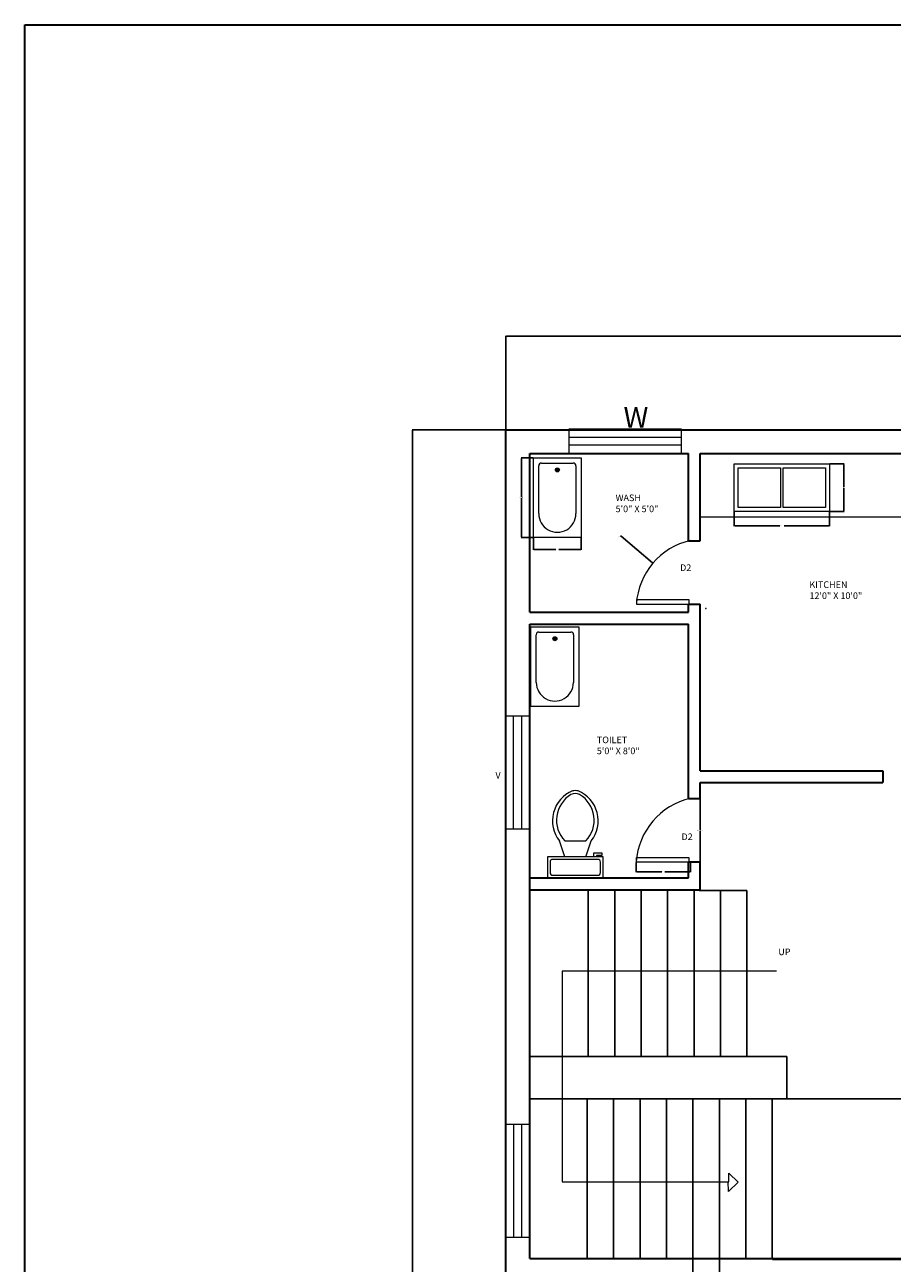
# Model space of a CAD drawing. Units: inches. Extents: x 65 to 1274, y 42 to 1041.
# Tile 2 of 6: x 65 to 393, y 573 to 1041. Entities that reach past the tile are written whole.
import ezdxf

# ---------------------------------------------------------------- set-up
doc = ezdxf.new("R2010")
doc.units = ezdxf.units.IN
for name, color, linetype, lineweight in [('A-ANNO-DIMS', 2, 'Continuous', 18), ('A-ANNO-SYMB', 7, 'Continuous', 13), ('A-AREA-IDEN', 7, 'Continuous', 18), ('A-DOOR', 3, 'Continuous', 18), ('A-FLOR-CASE', 8, 'Continuous', 18), ('A-FLOR-FIXT', 9, 'Continuous', 18), ('A-FLOR-STRS', 2, 'Continuous', 25), ('A-GLAZ', 4, 'Continuous', 18), ('A-WALL', 7, 'Continuous', 35), ('Text', 7, 'Continuous', 18), ('Title Block', 7, 'Continuous', 35)]:
    doc.layers.add(name, color=color, linetype=linetype, lineweight=lineweight)
doc.styles.get("Standard").update_dxf_attribs({"font": 'arial.ttf'})
doc.dimstyles.get("Standard").update_dxf_attribs({"dimtxt": 0.18, "dimasz": 0.18, "dimexe": 0.18, "dimexo": 0.0625, "dimgap": 0.09, "dimtad": 0, "dimtih": 1, "dimtoh": 1, "dimdec": 4, "dimzin": 0, "dimdsep": 46, "dimtxsty": 'Standard', "dimcen": 0.09, "dimadec": 0, "dimazin": 0, "dimtfac": 1, "dimtdec": 4, "dimtofl": 0, "dimtmove": 0, "dimatfit": 3, "dimfxl": 1, "dimtolj": 1, "dimtzin": 0, "dimarcsym": 0})

# ---------------------------------------------------------------- blocks, each defined once
blk = doc.blocks.new('Wall Cabinet - 18 x 36 in front')
for p, q in [((17.5, -1.5), (17.5, -16.5)), ((18.5, -16.5), (18.5, -1.5))]:
    blk.add_line(p, q)
blk.add_lwpolyline([(0, -18), (0, 0), (36, 0), (36, -18)], close=True)
for points in [[(17.5, -16.5), (1.5, -16.5), (1.5, -1.5), (17.5, -1.5)], [(18.5, -1.5), (34.5, -1.5), (34.5, -16.5), (18.5, -16.5)]]:
    blk.add_lwpolyline(points)
blk = doc.blocks.new('Bath Tub - 26 x 60 in.')
for p, q in [((8, -18), (10, -18)), ((9, -17), (9, -19))]:
    blk.add_line(p, q)
blk.add_lwpolyline([(0, -36), (0, 0), (60, 0), (60, -36)], close=True)
for points in [[(4, -30), (4, -6)], [(6, -4), (42, -4)], [(42, -32), (6, -32)]]:
    blk.add_lwpolyline(points)
for radius in [1.5, 1]:
    blk.add_circle((9, -18), radius)
for centre, radius, start, end in [((5.75, -5.75), 1.77, 81.8699, 188.1301), ((42, -18), 14, 270, 90), ((5.75, -30.25), 1.77, 171.8699, 278.1301)]:
    blk.add_arc(centre, radius, start, end)
blk = doc.blocks.new('Toilet - top')
for p, q in [((9.5, -6), (9.5, -2)), ((-10, -8.5), (-8, -8.5)), ((-10, -9.5), (-10, -8.5)), ((-8, -8.5), (-8, -8)), ((-7, -8), (-7, -9.5)), ((-4, -8), (-6, -14)), ((4, -8), (6, -14)), ((-7, -9.5), (-10, -9.5)), ((4, -14), (-4, -14))]:
    blk.add_line(p, q)
blk.add_lwpolyline([(10.5, -8), (10.5, 0), (-10.5, 0), (-10.5, -8)], close=True)
for points in [[(-9.5, -2), (-9.5, -6)], [(8.5, -1), (-8.5, -1)], [(-8.5, -7), (8.5, -7)]]:
    blk.add_lwpolyline(points)
for centre, radius, start, end in [((-8.62, -1.88), 0.884, 81.8699, 188.1301), ((8.62, -1.88), 0.884, 351.8699, 98.1301), ((-8.62, -6.12), 0.884, 171.8699, 278.1301), ((8.62, -6.12), 0.884, 261.8699, 8.1301), ((3.52, -21.58), 12.17, 141.4691, 247.9714), ((4.2, -21.82), 11.33, 136.3677, 238.9468), ((-3.52, -21.58), 12.17, 292.0284, 38.5307), ((-4.2, -21.82), 11.33, 301.053, 43.6321), ((0, -27.88), 4, 245.7318, 294.2682), ((0, -29), 4, 254.8605, 285.1395)]:
    blk.add_arc(centre, radius, start, end)
blk = doc.blocks.new('WIN-43-DEEP-FRAME')
for p, q in [((9, 42.65), (0, 42.65)), ((0, 42.65), (0, 0)), ((3, 0), (3, 42.65)), ((6, 42.65), (6, 0)), ((9, 0), (9, 42.65)), ((0, 0), (9, 0))]:
    blk.add_line(p, q)
blk = doc.blocks.new('DOOR-SINGLE-24')
blk.add_lwpolyline([(19.83, 0), (0.13, 0), (0.13, 1.84), (19.83, 1.84)], close=True)
blk.add_arc((26.27, -1.53), 26.32, 102.6921, 176.3801)
blk = doc.blocks.new('*D26')
at = {"layer": 'A-ANNO-DIMS', "color": 0, "lineweight": -2, "transparency": 16777216}
for p, q in [((316.53, 748.64), (320.27, 748.64)), ((320.09, 748.46), (320.09, 736.75)), ((320.09, 724.68), (320.09, 736.39)), ((316.53, 724.5), (320.27, 724.5))]:
    blk.add_line(p, q, dxfattribs=at)
at = {"layer": 'A-ANNO-DIMS', "color": 0, "transparency": 16777216}
for points in [[(320.06, 748.46), (320.12, 748.46), (320.09, 748.64)], [(320.06, 724.68), (320.12, 724.68), (320.09, 724.5)]]:
    blk.add_solid(points, dxfattribs=at)
at = {"layer": 'Defpoints', "color": 0, "transparency": 16777216}
for p in [(316.47, 748.64), (320.09, 748.64), (316.47, 724.5)]:
    blk.add_point(p, dxfattribs=at)
at = {"layer": 'A-ANNO-DIMS', "color": 0, "transparency": 16777216, "insert": (320.09, 736.57), "char_height": 0.18, "attachment_point": 5}
blk.add_mtext('\\A1;SERVICE DOOR 24 TYP.', dxfattribs=at)
blk = doc.blocks.new('*D27')
at = {"layer": 'A-ANNO-DIMS', "color": 0, "lineweight": -2, "transparency": 16777216}
for p, q in [((295.99, 724.44), (295.99, 720.7)), ((316.47, 724.44), (316.47, 720.7)), ((296.17, 720.88), (305.7, 720.88)), ((316.29, 720.88), (306.76, 720.88))]:
    blk.add_line(p, q, dxfattribs=at)
at = {"layer": 'A-ANNO-DIMS', "color": 0, "transparency": 16777216}
for points in [[(296.17, 720.91), (296.17, 720.85), (295.99, 720.88)], [(316.29, 720.91), (316.29, 720.85), (316.47, 720.88)]]:
    blk.add_solid(points, dxfattribs=at)
at = {"layer": 'Defpoints', "color": 0, "transparency": 16777216}
for p in [(295.99, 724.5), (316.47, 724.5), (316.47, 720.88)]:
    blk.add_point(p, dxfattribs=at)
at = {"layer": 'A-ANNO-DIMS', "color": 0, "transparency": 16777216, "insert": (306.23, 720.88), "char_height": 0.18, "attachment_point": 5}
blk.add_mtext('\\A1;20 TYP.', dxfattribs=at)
blk = doc.blocks.new('*D32')
at = {"layer": 'A-ANNO-DIMS', "color": 0, "lineweight": -2, "transparency": 16777216}
for p, q in [((257.04, 877.45), (252.4, 877.45)), ((252.58, 877.27), (252.58, 862.56)), ((252.58, 847.5), (252.58, 862.2)), ((257.04, 847.32), (252.4, 847.32))]:
    blk.add_line(p, q, dxfattribs=at)
at = {"layer": 'A-ANNO-DIMS', "color": 0, "transparency": 16777216}
for points in [[(252.55, 877.27), (252.61, 877.27), (252.58, 877.45)], [(252.55, 847.5), (252.61, 847.5), (252.58, 847.32)]]:
    blk.add_solid(points, dxfattribs=at)
at = {"layer": 'Defpoints', "color": 0, "transparency": 16777216}
for p in [(257.1, 877.45), (252.58, 847.32), (257.1, 847.32)]:
    blk.add_point(p, dxfattribs=at)
at = {"layer": 'A-ANNO-DIMS', "color": 0, "transparency": 16777216, "insert": (252.58, 862.38), "char_height": 0.18, "attachment_point": 5}
blk.add_mtext('\\A1;TUB 30 TYP.', dxfattribs=at)
blk = doc.blocks.new('*D33')
at = {"layer": 'A-ANNO-DIMS', "color": 0, "lineweight": -2, "transparency": 16777216}
for p, q in [((257.1, 847.25), (257.1, 842.62)), ((275.18, 847.25), (275.18, 842.62)), ((257.28, 842.8), (265.62, 842.8)), ((275, 842.8), (266.66, 842.8))]:
    blk.add_line(p, q, dxfattribs=at)
at = {"layer": 'A-ANNO-DIMS', "color": 0, "transparency": 16777216}
for points in [[(257.28, 842.83), (257.28, 842.77), (257.1, 842.8)], [(275, 842.83), (275, 842.77), (275.18, 842.8)]]:
    blk.add_solid(points, dxfattribs=at)
at = {"layer": 'Defpoints', "color": 0, "transparency": 16777216}
for p in [(257.1, 847.32), (275.18, 847.32), (275.18, 842.8)]:
    blk.add_point(p, dxfattribs=at)
at = {"layer": 'A-ANNO-DIMS', "color": 0, "transparency": 16777216, "insert": (266.14, 842.8), "char_height": 0.18, "attachment_point": 5}
blk.add_mtext('\\A1;18 TYP.', dxfattribs=at)
blk = doc.blocks.new('*D50')
at = {"layer": 'A-ANNO-DIMS', "color": 0, "lineweight": -2, "transparency": 16777216}
for p, q in [((333.04, 857.11), (333.04, 851.59)), ((369.04, 857.11), (369.04, 851.59)), ((333.22, 851.77), (350.25, 851.77)), ((368.86, 851.77), (351.84, 851.77))]:
    blk.add_line(p, q, dxfattribs=at)
at = {"layer": 'A-ANNO-DIMS', "color": 0, "transparency": 16777216}
for points in [[(333.22, 851.8), (333.22, 851.74), (333.04, 851.77)], [(368.86, 851.8), (368.86, 851.74), (369.04, 851.77)]]:
    blk.add_solid(points, dxfattribs=at)
at = {"layer": 'Defpoints', "color": 0, "transparency": 16777216}
for p in [(333.04, 857.17), (369.04, 857.17), (369.04, 851.77)]:
    blk.add_point(p, dxfattribs=at)
at = {"layer": 'A-ANNO-DIMS', "color": 0, "transparency": 16777216, "insert": (351.04, 851.77), "char_height": 0.18, "attachment_point": 5}
blk.add_mtext('\\A1;CABINET 36', dxfattribs=at)
blk = doc.blocks.new('*D51')
at = {"layer": 'A-ANNO-DIMS', "color": 0, "lineweight": -2, "transparency": 16777216}
for p, q in [((369.11, 875.17), (374.62, 875.17)), ((374.44, 874.99), (374.44, 866.35)), ((374.44, 857.35), (374.44, 865.99)), ((369.11, 857.17), (374.62, 857.17))]:
    blk.add_line(p, q, dxfattribs=at)
at = {"layer": 'A-ANNO-DIMS', "color": 0, "transparency": 16777216}
for points in [[(374.41, 874.99), (374.47, 874.99), (374.44, 875.17)], [(374.41, 857.35), (374.47, 857.35), (374.44, 857.17)]]:
    blk.add_solid(points, dxfattribs=at)
at = {"layer": 'Defpoints', "color": 0, "transparency": 16777216}
for p in [(369.04, 875.17), (374.44, 875.17), (369.04, 857.17)]:
    blk.add_point(p, dxfattribs=at)
at = {"layer": 'A-ANNO-DIMS', "color": 0, "transparency": 16777216, "insert": (374.44, 866.17), "char_height": 0.18, "attachment_point": 5}
blk.add_mtext('\\A1;18', dxfattribs=at)
blk = doc.blocks.new('*D52')
at = {"layer": 'A-ANNO-DIMS', "color": 0, "lineweight": -2, "transparency": 16777216}
for p, q in [((246.69, 888.16), (246.69, 923.68)), ((246.87, 923.5), (438.4, 923.5)), ((630.51, 923.5), (438.98, 923.5)), ((630.69, 888.16), (630.69, 923.68))]:
    blk.add_line(p, q, dxfattribs=at)
at = {"layer": 'A-ANNO-DIMS', "color": 0, "transparency": 16777216}
for points in [[(246.87, 923.53), (246.87, 923.47), (246.69, 923.5)], [(630.51, 923.53), (630.51, 923.47), (630.69, 923.5)]]:
    blk.add_solid(points, dxfattribs=at)
at = {"layer": 'Defpoints', "color": 0, "transparency": 16777216}
for p in [(630.69, 923.5), (246.69, 888.1), (630.69, 888.1)]:
    blk.add_point(p, dxfattribs=at)
at = {"layer": 'A-ANNO-DIMS', "color": 0, "transparency": 16777216, "insert": (438.69, 923.5), "char_height": 0.18, "attachment_point": 5}
blk.add_mtext('\\A1;384', dxfattribs=at)
blk = doc.blocks.new('*D53')
at = {"layer": 'A-ANNO-DIMS', "color": 0, "lineweight": -2, "transparency": 16777216}
for p, q in [((246.62, 888.1), (211.23, 888.1)), ((211.41, 887.92), (211.41, 559.78)), ((211.41, 231.28), (211.41, 559.42)), ((246.62, 231.1), (211.23, 231.1))]:
    blk.add_line(p, q, dxfattribs=at)
at = {"layer": 'A-ANNO-DIMS', "color": 0, "transparency": 16777216}
for points in [[(211.38, 887.92), (211.44, 887.92), (211.41, 888.1)], [(211.38, 231.28), (211.44, 231.28), (211.41, 231.1)]]:
    blk.add_solid(points, dxfattribs=at)
at = {"layer": 'Defpoints', "color": 0, "transparency": 16777216}
for p in [(211.41, 888.1), (246.69, 888.1), (246.69, 231.1)]:
    blk.add_point(p, dxfattribs=at)
at = {"layer": 'A-ANNO-DIMS', "color": 0, "transparency": 16777216, "insert": (211.41, 559.6), "char_height": 0.18, "attachment_point": 5}
blk.add_mtext('\\A1;657', dxfattribs=at)
blk = doc.blocks.new('*D62')
at = {"layer": 'A-ANNO-DIMS', "color": 0, "lineweight": -2, "transparency": 16777216}
for p, q in [((347.47, 635.01), (666.07, 635.01)), ((665.89, 634.83), (665.89, 604.83)), ((665.89, 574.45), (665.89, 604.46)), ((347.47, 574.27), (666.07, 574.27))]:
    blk.add_line(p, q, dxfattribs=at)
at = {"layer": 'A-ANNO-DIMS', "color": 0, "transparency": 16777216}
for points in [[(665.86, 634.83), (665.92, 634.83), (665.89, 635.01)], [(665.86, 574.45), (665.92, 574.45), (665.89, 574.27)]]:
    blk.add_solid(points, dxfattribs=at)
at = {"layer": 'Defpoints', "color": 0, "transparency": 16777216}
for p in [(347.41, 635.01), (665.89, 635.01), (347.41, 574.27)]:
    blk.add_point(p, dxfattribs=at)
at = {"layer": 'A-ANNO-DIMS', "color": 0, "transparency": 16777216, "insert": (665.89, 604.64), "char_height": 0.18, "attachment_point": 5}
blk.add_mtext('\\A1;60.74', dxfattribs=at)
blk = doc.blocks.new('*D63')
at = {"layer": 'A-ANNO-DIMS', "color": 0, "lineweight": -2, "transparency": 16777216}
for p, q in [((317.41, 574.21), (317.41, 195.72)), ((327.41, 574.21), (327.41, 195.72)), ((317.59, 195.9), (322.2, 195.9)), ((327.23, 195.9), (322.62, 195.9))]:
    blk.add_line(p, q, dxfattribs=at)
at = {"layer": 'A-ANNO-DIMS', "color": 0, "transparency": 16777216}
for points in [[(317.59, 195.93), (317.59, 195.87), (317.41, 195.9)], [(327.23, 195.93), (327.23, 195.87), (327.41, 195.9)]]:
    blk.add_solid(points, dxfattribs=at)
at = {"layer": 'Defpoints', "color": 0, "transparency": 16777216}
for p in [(317.41, 574.27), (327.41, 574.27), (327.41, 195.9)]:
    blk.add_point(p, dxfattribs=at)
at = {"layer": 'A-ANNO-DIMS', "color": 0, "transparency": 16777216, "insert": (322.41, 195.9), "char_height": 0.18, "attachment_point": 5}
blk.add_mtext('\\A1;10', dxfattribs=at)
blk = doc.blocks.new('*D79')
at = {"layer": 'A-ANNO-DIMS', "color": 0, "lineweight": -2, "transparency": 16777216}
for p, q in [((290.06, 847.85), (290.24, 847.85)), ((290.24, 847.85), (302.11, 837.72)), ((322.18, 820.52), (322.36, 820.52)), ((322.27, 820.43), (322.27, 820.61))]:
    blk.add_line(p, q, dxfattribs=at)
at = {"layer": 'A-ANNO-DIMS', "color": 0, "transparency": 16777216}
blk.add_solid([(302.13, 837.74), (302.09, 837.69), (302.25, 837.6)], dxfattribs=at)
at = {"layer": 'Defpoints', "color": 0, "transparency": 16777216}
for p in [(302.25, 837.6), (322.27, 820.52)]:
    blk.add_point(p, dxfattribs=at)
at = {"layer": 'A-ANNO-DIMS', "color": 0, "transparency": 16777216, "insert": (289.38, 847.85), "char_height": 0.18, "attachment_point": 5}
blk.add_mtext('\\A1;2X R26.32', dxfattribs=at)

msp = doc.modelspace()

# ---------------------------------------------------------------- linework, layer by layer
at = {"layer": 'A-ANNO-SYMB'}
for p, q in [((349.0318, 683.2572), (267.9966, 683.2572)), ((267.9966, 683.2572), (267.9966, 603.565)), ((330.9282, 603.565), (330.9282, 606.9116)), ((330.9282, 606.9116), (334.457, 603.5371)), ((267.9966, 603.565), (330.9282, 603.565)), ((330.9115, 599.9938), (330.7427, 603.7058)), ((334.457, 603.5371), (330.9115, 599.9938))]:
    msp.add_line(p, q, dxfattribs=at)
at = {"layer": 'A-FLOR-CASE'}
msp.add_line((320.1872, 855.1013), (440.1872, 855.1013), dxfattribs=at)
at = {"layer": 'A-FLOR-STRS'}
for p, q in [((277.8365, 713.8438), (277.8365, 650.9516)), ((287.8365, 713.8438), (287.8365, 650.9516)), ((297.8365, 713.8438), (297.8365, 650.9516)), ((307.8365, 713.8438), (307.8365, 650.9516)), ((317.8365, 713.8438), (317.8365, 650.9516)), ((319.7329, 713.8438), (337.8365, 713.8438)), ((327.8365, 713.8438), (327.8365, 650.9516)), ((337.8365, 713.8438), (337.8365, 650.9516)), ((255.6872, 650.9516), (352.9229, 650.9516)), ((352.9229, 650.9516), (352.9229, 635.0131)), ((352.9229, 635.0131), (255.6872, 635.0131)), ((277.4055, 635.0131), (277.4055, 574.2747)), ((287.4055, 635.0131), (287.4055, 574.2747)), ((297.4055, 635.0131), (297.4055, 574.2747)), ((307.4055, 635.0131), (307.4055, 574.2747)), ((317.4055, 635.0131), (317.4055, 574.2747)), ((327.4055, 635.0131), (327.4055, 574.2747)), ((337.4055, 635.0131), (337.4055, 574.2747)), ((347.4055, 635.0131), (347.4055, 574.2747))]:
    msp.add_line(p, q, dxfattribs=at)
at = {"layer": 'A-WALL'}
for p, q in [((246.6872, 231.1013), (246.6872, 888.1013)), ((246.6872, 888.1013), (630.6872, 888.1013)), ((255.6872, 879.1013), (315.6872, 879.1013)), ((255.6872, 819.1013), (255.6872, 879.1013)), ((315.6872, 846.1013), (315.6872, 879.1013)), ((315.6872, 846.1013), (315.6872, 879.1013)), ((320.1872, 846.1013), (320.1872, 879.1013)), ((320.1872, 879.1013), (464.1872, 879.1013)), ((315.6872, 846.1013), (320.1872, 846.1013)), ((315.6872, 819.1013), (315.6872, 822.1013)), ((315.6872, 822.1013), (320.1872, 822.1013)), ((315.6872, 819.1013), (315.6872, 822.1013)), ((320.1872, 759.1013), (320.1872, 822.1013)), ((255.6872, 819.1013), (315.6872, 819.1013)), ((320.1872, 814.6013), (320.1872, 819.1013)), ((255.6872, 814.6013), (315.6872, 814.6013)), ((255.6872, 574.6013), (255.6872, 814.6013)), ((315.6872, 748.6013), (315.6872, 814.6013)), ((320.1872, 759.1013), (389.1872, 759.1013)), ((389.1872, 759.1013), (389.1872, 754.6013)), ((320.1872, 754.6013), (389.1872, 754.6013)), ((320.1872, 748.6013), (320.1872, 754.6013)), ((315.6872, 748.6013), (320.1872, 748.6013)), ((315.6872, 718.6013), (315.6872, 724.6013)), ((315.6872, 724.6013), (320.1872, 724.6013)), ((320.1872, 714.1013), (320.1872, 724.6013)), ((255.6872, 718.6013), (315.6872, 718.6013)), ((255.6872, 714.1013), (320.1872, 714.1013)), ((255.6872, 574.6013), (441.6872, 574.6013))]:
    msp.add_line(p, q, dxfattribs=at)
at = {"layer": 'Title Block'}
msp.add_lwpolyline([(64.7421, 1041.286), (1273.976, 1041.286), (1273.976, 41.6396), (64.7421, 41.6396)], close=True, dxfattribs=at)

# ---------------------------------------------------------------- block references
at = {"layer": 'A-DOOR'}
for p in [(296.0064, 822.0505), (295.986, 724.499)]:
    msp.add_blockref('DOOR-SINGLE-24', p, dxfattribs=at)
at = {"layer": 'A-FLOR-CASE'}
msp.add_blockref('Wall Cabinet - 18 x 36 in front', (333.043, 875.1694), dxfattribs=at)
at = {"layer": 'A-FLOR-FIXT', "xscale": 0.5021616587859374, "yscale": 0.5021616587859374, "zscale": 0.5021616587859374, "rotation": 270}
for p in [(275.1788, 877.4464), (274.2366, 813.5706)]:
    msp.add_blockref('Bath Tub - 26 x 60 in.', p, dxfattribs=at)
at = {"layer": 'A-FLOR-FIXT', "rotation": 180}
msp.add_blockref('Toilet - top', (272.9251, 718.5865), dxfattribs=at)
at = {"layer": 'A-GLAZ'}
for p, rotation in [((270.476, 888.2993), 269.9999999999994), ((255.6126, 779.7517), 180), ((255.621, 625.3174), 180)]:
    msp.add_blockref('WIN-43-DEEP-FRAME', p, dxfattribs=dict(at, rotation=rotation))

# ---------------------------------------------------------------- texts
at = {"layer": 'A-AREA-IDEN', "char_height": 2.5, "attachment_point": 1}
for s, width, insert in [('WASH\\P5\'0" X 5\'0"', 20.053164, (288.1552, 863.5853)), ('KITCHEN\\P12\'0" X 10\'0"', 36.578531, (361.4522, 830.7528)), ('TOILET\\P5\'0" X 8\'0" ', 18.101103, (281.0621, 772.0325))]:
    msp.add_mtext_dynamic_manual_height_columns(s, width=width, gutter_width=12.5, heights=[0], dxfattribs=dict(at, insert=insert))
at = {"layer": 'Text', "attachment_point": 1}
for s, width, gutter_width, insert, char_height in [('W', 96.254197, 39.1027, (291.1598, 896.645), 7.8205), ('D2', 14.123415, 12.5, (312.5465, 837.1667), 2.5), ('V', 5.099062, 12.5, (242.7261, 758.6419), 2.5), ('D2', 14.019907, 12.5, (313.0605, 735.3946), 2.5), ('UP', 18.012995, 12.5, (349.6789, 691.8471), 2.5)]:
    msp.add_mtext_dynamic_manual_height_columns(s, width=width, gutter_width=gutter_width, heights=[0], dxfattribs=dict(at, insert=insert, char_height=char_height))

# ---------------------------------------------------------------- dimensions: what is measured, and where the dimension line sits
at = {"layer": 'A-ANNO-DIMS'}
for base, p1, p2, picture, middle in [((630.6872, 923.4993), (246.6872, 888.1013), (630.6872, 888.1013), '*D52', (438.6872, 923.4993)), ((327.4055, 195.9013), (317.4055, 574.2747), (327.4055, 574.2747), '*D63', (322.4055, 195.9013))]:
    dim = msp.add_linear_dim(base=base, p1=p1, p2=p2, dimstyle='Standard', override={"dimdec": 0, "dimlfac": 1, "dimrnd": 0, "dimzin": 0, "dimdsep": 46, "dimlunit": 2}, dxfattribs=at)
    dim.commit()
    dim.dimension.update_dxf_attribs({"geometry": picture, "text_midpoint": middle})
for base, p1, p2, override, picture, middle in [((211.4126, 888.1013), (246.6872, 231.1013), (246.6872, 888.1013), {"dimdec": 0, "dimlfac": 1, "dimrnd": 0, "dimzin": 0, "dimdsep": 46, "dimlunit": 2}, '*D53', (211.4126, 559.6013)), ((374.443, 875.1694), (369.043, 857.1694), (369.043, 875.1694), {"dimdec": 0, "dimlfac": 1, "dimrnd": 0, "dimzin": 0, "dimdsep": 46, "dimlunit": 2}, '*D51', (374.443, 866.1694)), ((665.8872, 635.0131), (347.4055, 574.2747), (347.4055, 635.0131), {"dimdec": 2, "dimlfac": 1, "dimrnd": 0, "dimzin": 0, "dimdsep": 46, "dimlunit": 2}, '*D62', (665.8872, 604.6439))]:
    dim = msp.add_linear_dim(base=base, p1=p1, p2=p2, angle=90, dimstyle='Standard', override=override, dxfattribs=at)
    dim.commit()
    dim.dimension.update_dxf_attribs({"geometry": picture, "text_midpoint": middle})
for base, p1, p2, angle, text, picture, middle in [((252.5815, 847.3167), (257.101, 877.4464), (257.101, 847.3167), 270, 'TUB <> TYP.', '*D32', (252.5815, 862.3815)), ((320.0914, 748.6438), (316.4696, 724.4986), (316.4696, 748.6438), 90, 'SERVICE DOOR <> TYP.', '*D26', (320.0914, 736.5712))]:
    dim = msp.add_linear_dim(base=base, p1=p1, p2=p2, angle=angle, text=text, dimstyle='Standard', override={"dimdec": 0, "dimlfac": 1, "dimrnd": 0, "dimzin": 0, "dimdsep": 46, "dimlunit": 2}, dxfattribs=at)
    dim.commit()
    dim.dimension.update_dxf_attribs({"geometry": picture, "text_midpoint": middle})
for base, p1, p2, text, picture, middle in [((369.043, 851.7694), (333.043, 857.1694), (369.043, 857.1694), 'CABINET <>', '*D50', (351.043, 851.7694)), ((275.1788, 842.7972), (257.101, 847.3167), (275.1788, 847.3167), '<> TYP.', '*D33', (266.1399, 842.7972)), ((316.4696, 720.8769), (295.986, 724.4986), (316.4696, 724.4986), '<> TYP.', '*D27', (306.2278, 720.8769))]:
    dim = msp.add_linear_dim(base=base, p1=p1, p2=p2, text=text, dimstyle='Standard', override={"dimdec": 0, "dimlfac": 1, "dimrnd": 0, "dimzin": 0, "dimdsep": 46, "dimlunit": 2}, dxfattribs=at)
    dim.commit()
    dim.dimension.update_dxf_attribs({"geometry": picture, "text_midpoint": middle})
dim = msp.add_radius_dim(center=(322.2726, 820.5198), mpoint=(302.2491, 837.5999), text='2X <>', dimstyle='Standard', override={"dimdec": 2, "dimlfac": 1, "dimrnd": 0, "dimzin": 0, "dimdsep": 46, "dimlunit": 2}, dxfattribs=at)
dim.commit()
dim.dimension.update_dxf_attribs({"geometry": '*D79', "text_midpoint": (289.3812, 847.848), "dimtype": 164})

doc.saveas('drawing.dxf')
